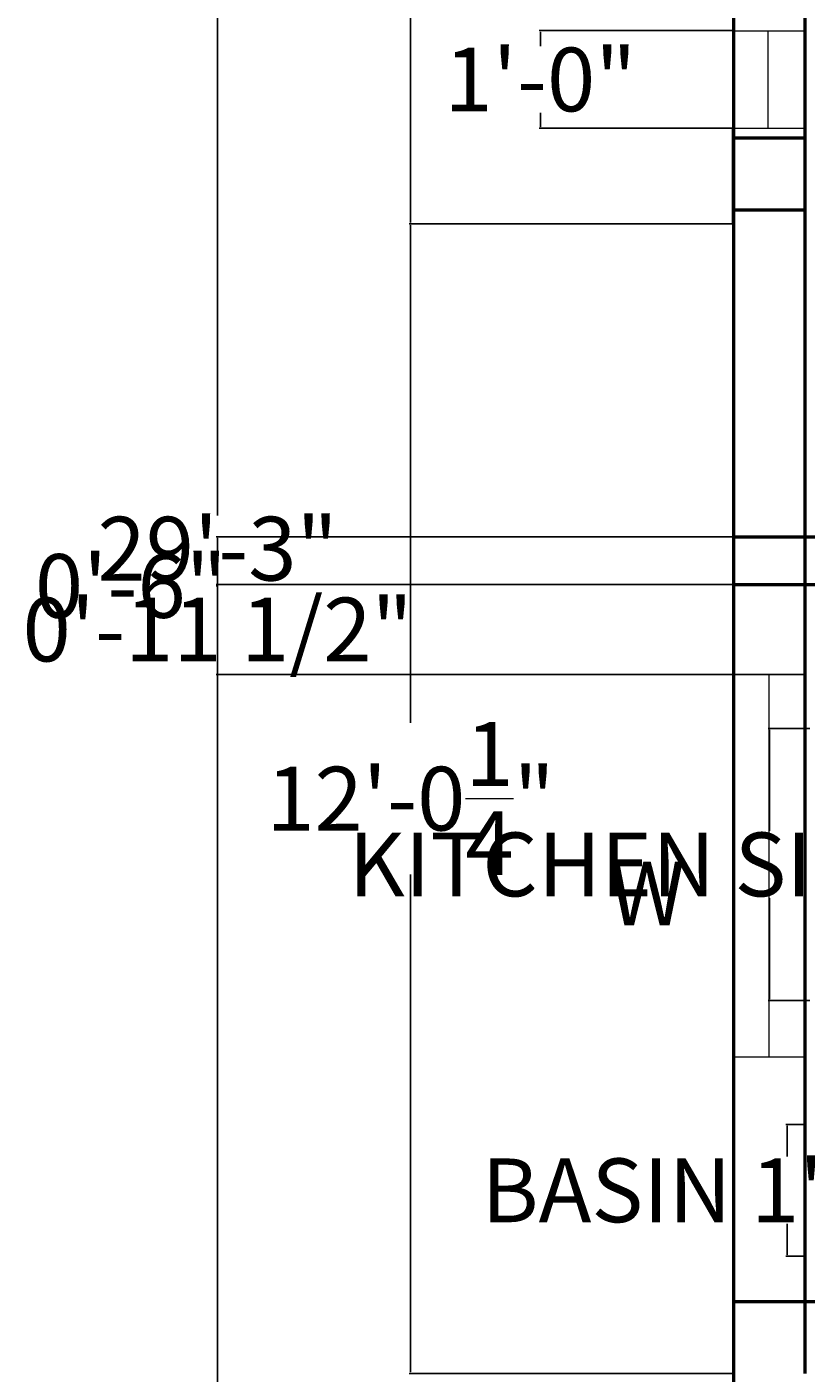
# Model space of a CAD drawing. Units: inches. Extents: x 1305 to 1889, y -508 to -5.
# Tile 2 of 8: x 1305 to 1403, y -389 to -220. Entities that reach past the tile are written whole.
import ezdxf

# ---------------------------------------------------------------- set-up
doc = ezdxf.new("R2010")
doc.units = ezdxf.units.IN
doc.header["$MEASUREMENT"] = 0
for name, color, linetype, lineweight in [('A-ANNO-DIMS', 2, 'Continuous', 18), ('A-ANNO-TEXT', 7, 'Continuous', 18), ('A-COLS', 7, 'Continuous', 50), ('A-GLAZ', 4, 'Continuous', 18), ('A-WALL', 7, 'Continuous', 50)]:
    doc.layers.add(name, color=color, linetype=linetype, lineweight=lineweight)
doc.styles.get("Standard").update_dxf_attribs({"font": 'arial.ttf', "height": 8})
doc.dimstyles.get("Standard").update_dxf_attribs({"dimtxt": 0.18, "dimasz": 0.18, "dimexe": 0.18, "dimexo": 0.0625, "dimgap": 0.09, "dimtad": 0, "dimtih": 1, "dimtoh": 1, "dimzin": 0, "dimdsep": 46, "dimlunit": 4, "dimtxsty": 'Standard', "dimcen": 0.09, "dimadec": 0, "dimazin": 0, "dimtfac": 1, "dimtofl": 0, "dimtmove": 0, "dimatfit": 3, "dimfxl": 1, "dimtolj": 1, "dimtzin": 0, "dimarcsym": 0})

# ---------------------------------------------------------------- blocks, each defined once
blk = doc.blocks.new('*D20')
at = {"layer": 'A-ANNO-DIMS', "color": 0, "lineweight": -2, "transparency": 16777216}
for p, q in [((1394.01, -110.24), (1353.36, -110.24)), ((1353.54, -110.42), (1353.54, -168.1)), ((1353.54, -244.8), (1353.54, -187.12)), ((1394.01, -244.98), (1353.36, -244.98))]:
    blk.add_line(p, q, dxfattribs=at)
at = {"layer": 'A-ANNO-DIMS', "color": 0, "transparency": 16777216}
for points in [[(1353.51, -110.42), (1353.57, -110.42), (1353.54, -110.24)], [(1353.51, -244.8), (1353.57, -244.8), (1353.54, -244.98)]]:
    blk.add_solid(points, dxfattribs=at)
at = {"layer": 'Defpoints', "color": 0, "transparency": 16777216}
for p in [(1394.07, -110.24), (1353.54, -244.98), (1394.07, -244.98)]:
    blk.add_point(p, dxfattribs=at)
at = {"layer": 'A-ANNO-DIMS', "color": 0, "transparency": 16777216, "insert": (1353.54, -177.61), "char_height": 8, "attachment_point": 5}
blk.add_mtext('\\A1;11\'-2{\\H1x;\\S3/4;}"', dxfattribs=at)
blk = doc.blocks.new('*D21')
at = {"layer": 'A-ANNO-DIMS', "color": 0, "lineweight": -2, "transparency": 16777216}
for p, q in [((1394.01, -244.98), (1353.36, -244.98)), ((1353.54, -245.16), (1353.54, -307.6)), ((1353.54, -389.06), (1353.54, -326.62)), ((1394.01, -389.24), (1353.36, -389.24))]:
    blk.add_line(p, q, dxfattribs=at)
at = {"layer": 'A-ANNO-DIMS', "color": 0, "transparency": 16777216}
for points in [[(1353.51, -245.16), (1353.57, -245.16), (1353.54, -244.98)], [(1353.51, -389.06), (1353.57, -389.06), (1353.54, -389.24)]]:
    blk.add_solid(points, dxfattribs=at)
at = {"layer": 'Defpoints', "color": 0, "transparency": 16777216}
for p in [(1394.07, -244.98), (1353.54, -389.24), (1394.07, -389.24)]:
    blk.add_point(p, dxfattribs=at)
at = {"layer": 'A-ANNO-DIMS', "color": 0, "transparency": 16777216, "insert": (1353.54, -317.11), "char_height": 8, "attachment_point": 5}
blk.add_mtext('\\A1;12\'-0{\\H1x;\\S1/4;}"', dxfattribs=at)
blk = doc.blocks.new('WIN-48IN')
for p, q in [((0, 9), (0, 0)), ((48, 9), (48, 0)), ((48, 4.5), (0, 4.5))]:
    blk.add_line(p, q)
blk = doc.blocks.new('COL-9X9')
blk.add_lwpolyline([(0, 0), (9, 0), (9, 9), (0, 9)], close=True)
blk = doc.blocks.new('*D34')
at = {"layer": 'A-ANNO-DIMS', "color": 0, "lineweight": -2, "transparency": 16777216}
for p, q in [((1403.25, -358), (1400.66, -358)), ((1400.84, -358.18), (1400.84, -362.04)), ((1400.84, -374.35), (1400.84, -370.49)), ((1403.25, -374.53), (1400.66, -374.53))]:
    blk.add_line(p, q, dxfattribs=at)
at = {"layer": 'A-ANNO-DIMS', "color": 0, "transparency": 16777216}
for points in [[(1400.81, -358.18), (1400.87, -358.18), (1400.84, -358)], [(1400.81, -374.35), (1400.87, -374.35), (1400.84, -374.53)]]:
    blk.add_solid(points, dxfattribs=at)
at = {"layer": 'Defpoints', "color": 0, "transparency": 16777216}
for p in [(1403.32, -358), (1400.84, -374.53), (1403.32, -374.53)]:
    blk.add_point(p, dxfattribs=at)
at = {"layer": 'A-ANNO-DIMS', "color": 0, "transparency": 16777216, "insert": (1400.84, -366.27), "char_height": 8, "attachment_point": 5}
blk.add_mtext('\\A1;BASIN 1\'-4 1/2"', dxfattribs=at)
blk = doc.blocks.new('*D44')
at = {"layer": 'A-ANNO-DIMS', "color": 0, "lineweight": -2, "transparency": 16777216}
for p, q in [((1403.68, -308.29), (1398.44, -308.29)), ((1398.62, -308.47), (1398.62, -321.14)), ((1398.62, -342.27), (1398.62, -329.59)), ((1403.68, -342.45), (1398.44, -342.45))]:
    blk.add_line(p, q, dxfattribs=at)
at = {"layer": 'A-ANNO-DIMS', "color": 0, "transparency": 16777216}
for points in [[(1398.59, -308.47), (1398.65, -308.47), (1398.62, -308.29)], [(1398.59, -342.27), (1398.65, -342.27), (1398.62, -342.45)]]:
    blk.add_solid(points, dxfattribs=at)
at = {"layer": 'Defpoints', "color": 0, "transparency": 16777216}
for p in [(1403.74, -308.29), (1398.62, -342.45), (1403.74, -342.45)]:
    blk.add_point(p, dxfattribs=at)
at = {"layer": 'A-ANNO-DIMS', "color": 0, "transparency": 16777216, "insert": (1398.62, -325.37), "char_height": 8, "attachment_point": 5}
blk.add_mtext('\\A1;KITCHEN SINK 2\'-10"', dxfattribs=at)
blk = doc.blocks.new('*D51')
at = {"layer": 'A-ANNO-DIMS', "color": 0, "lineweight": -2, "transparency": 16777216}
for p, q in [((1394.01, -110.24), (1329.13, -110.24)), ((1329.31, -110.42), (1329.31, -281.56)), ((1329.31, -461.06), (1329.31, -289.92)), ((1394.01, -461.24), (1329.13, -461.24))]:
    blk.add_line(p, q, dxfattribs=at)
at = {"layer": 'A-ANNO-DIMS', "color": 0, "transparency": 16777216}
for points in [[(1329.28, -110.42), (1329.34, -110.42), (1329.31, -110.24)], [(1329.28, -461.06), (1329.34, -461.06), (1329.31, -461.24)]]:
    blk.add_solid(points, dxfattribs=at)
at = {"layer": 'Defpoints', "color": 0, "transparency": 16777216}
for p in [(1394.07, -110.24), (1329.31, -461.24), (1394.07, -461.24)]:
    blk.add_point(p, dxfattribs=at)
at = {"layer": 'A-ANNO-DIMS', "color": 0, "transparency": 16777216, "insert": (1329.31, -285.74), "char_height": 8, "attachment_point": 5}
blk.add_mtext('\\A1;29\'-3"', dxfattribs=at)
blk = doc.blocks.new('*D62')
at = {"layer": 'A-ANNO-DIMS', "color": 0, "lineweight": -2, "transparency": 16777216}
for p, q in [((1505.01, -284.24), (1329.13, -284.24)), ((1329.31, -284.42), (1329.31, -290.06)), ((1505.01, -290.24), (1329.13, -290.24)), ((1329.31, -290.42), (1329.13, -290.42)), ((1329.31, -290.24), (1329.31, -290.42))]:
    blk.add_line(p, q, dxfattribs=at)
at = {"layer": 'A-ANNO-DIMS', "color": 0, "transparency": 16777216}
for points in [[(1329.28, -284.42), (1329.34, -284.42), (1329.31, -284.24)], [(1329.28, -290.06), (1329.34, -290.06), (1329.31, -290.24)]]:
    blk.add_solid(points, dxfattribs=at)
at = {"layer": 'Defpoints', "color": 0, "transparency": 16777216}
for p in [(1505.07, -284.24), (1329.31, -290.24), (1505.07, -290.24)]:
    blk.add_point(p, dxfattribs=at)
at = {"layer": 'A-ANNO-DIMS', "color": 0, "transparency": 16777216, "insert": (1318.41, -290.42), "char_height": 8, "attachment_point": 5}
blk.add_mtext('\\A1;0\'-6"', dxfattribs=at)
blk = doc.blocks.new('*D66')
at = {"layer": 'A-ANNO-DIMS', "color": 0, "lineweight": -2, "transparency": 16777216}
for p, q in [((1394.01, -290.24), (1329.13, -290.24)), ((1329.31, -290.42), (1329.31, -291.67)), ((1329.31, -301.37), (1329.31, -300.12)), ((1403.01, -301.55), (1329.13, -301.55))]:
    blk.add_line(p, q, dxfattribs=at)
at = {"layer": 'A-ANNO-DIMS', "color": 0, "transparency": 16777216}
for points in [[(1329.28, -290.42), (1329.34, -290.42), (1329.31, -290.24)], [(1329.28, -301.37), (1329.34, -301.37), (1329.31, -301.55)]]:
    blk.add_solid(points, dxfattribs=at)
at = {"layer": 'Defpoints', "color": 0, "transparency": 16777216}
for p in [(1394.07, -290.24), (1329.31, -301.55), (1403.07, -301.55)]:
    blk.add_point(p, dxfattribs=at)
at = {"layer": 'A-ANNO-DIMS', "color": 0, "transparency": 16777216, "insert": (1329.31, -295.89), "char_height": 8, "attachment_point": 5}
blk.add_mtext('\\A1;0\'-11 1/2"', dxfattribs=at)
blk = doc.blocks.new('*D73')
at = {"layer": 'A-ANNO-DIMS', "color": 0, "lineweight": -2, "transparency": 16777216}
for p, q in [((1394.01, -220.73), (1369.67, -220.73)), ((1369.85, -220.91), (1369.85, -222.68)), ((1369.85, -232.8), (1369.85, -231.03)), ((1394.01, -232.98), (1369.67, -232.98))]:
    blk.add_line(p, q, dxfattribs=at)
at = {"layer": 'A-ANNO-DIMS', "color": 0, "transparency": 16777216}
for points in [[(1369.82, -220.91), (1369.88, -220.91), (1369.85, -220.73)], [(1369.82, -232.8), (1369.88, -232.8), (1369.85, -232.98)]]:
    blk.add_solid(points, dxfattribs=at)
at = {"layer": 'Defpoints', "color": 0, "transparency": 16777216}
for p in [(1369.85, -220.73), (1394.07, -220.73), (1394.07, -232.98)]:
    blk.add_point(p, dxfattribs=at)
at = {"layer": 'A-ANNO-DIMS', "color": 0, "transparency": 16777216, "insert": (1369.85, -226.86), "char_height": 8, "attachment_point": 5}
blk.add_mtext('\\A1;1\'-0"', dxfattribs=at)

msp = doc.modelspace()

# ---------------------------------------------------------------- linework, layer by layer
at = {"layer": 'A-GLAZ'}
for p, q in [((1394.074, -220.734), (1403.074, -220.734)), ((1398.425, -220.734), (1398.425, -232.978)), ((1394.074, -232.978), (1403.074, -232.978))]:
    msp.add_line(p, q, dxfattribs=at)
at = {"layer": 'A-WALL'}
for p, q in [((1394.074, -110.239), (1394.074, -461.239)), ((1403.074, -110.239), (1403.074, -389.239)), ((1394.074, -244.978), (1394.074, -232.978)), ((1403.074, -232.978), (1403.074, -244.978)), ((1394.074, -284.239), (1505.074, -284.239)), ((1394.074, -290.239), (1505.074, -290.239)), ((1394.074, -380.239), (1547.074, -380.239))]:
    msp.add_line(p, q, dxfattribs=at)

# ---------------------------------------------------------------- block references
at = {"layer": 'A-COLS'}
msp.add_blockref('COL-9X9', (1394.108, -243.228), dxfattribs=at)
at = {"layer": 'A-GLAZ', "rotation": 269.9999999999999}
msp.add_blockref('WIN-48IN', (1394.074, -301.548), dxfattribs=at)

# ---------------------------------------------------------------- texts
at = {"layer": 'A-ANNO-TEXT', "insert": (1378.42, -325.014), "char_height": 8, "attachment_point": 1}
msp.add_mtext_dynamic_manual_height_columns('W', width=13.3749, gutter_width=40, heights=[0], dxfattribs=at)

# ---------------------------------------------------------------- dimensions: what is measured, and where the dimension line sits
at = {"layer": 'A-ANNO-DIMS'}
for base, p1, p2, override, picture, middle in [((1329.31, -461.239), (1394.074, -110.239), (1394.074, -461.239), {"dimdec": 1, "dimlfac": 1, "dimrnd": 0, "dimzin": 1, "dimdsep": 46, "dimlunit": 4, "dimfrac": 2}, '*D51', (1329.31, -285.739)), ((1353.535, -244.978), (1394.074, -110.239), (1394.074, -244.978), {"dimclrd": 0, "dimclre": 0, "dimclrt": 0}, '*D20', (1353.535, -177.608)), ((1369.849, -220.734), (1394.074, -232.978), (1394.074, -220.734), {"dimdec": 1, "dimlfac": 1, "dimrnd": 0, "dimzin": 1, "dimdsep": 46, "dimlunit": 4, "dimfrac": 2}, '*D73', (1369.849, -226.856)), ((1353.535, -389.239), (1394.074, -244.978), (1394.074, -389.239), {"dimclrd": 0, "dimclre": 0, "dimclrt": 0}, '*D21', (1353.535, -317.108)), ((1329.31, -301.547), (1394.074, -290.239), (1403.074, -301.547), {"dimdec": 1, "dimlfac": 1, "dimrnd": 0, "dimzin": 1, "dimdsep": 46, "dimlunit": 4, "dimfrac": 2}, '*D66', (1329.31, -295.893)), ((1329.31, -290.239), (1505.074, -284.239), (1505.074, -290.239), {"dimdec": 1, "dimlfac": 1, "dimrnd": 0, "dimzin": 1, "dimdsep": 46, "dimlunit": 4, "dimfrac": 2}, '*D62', (1318.407, -290.419))]:
    dim = msp.add_linear_dim(base=base, p1=p1, p2=p2, angle=90, dimstyle='Standard', override=override, dxfattribs=at)
    dim.commit()
    dim.dimension.update_dxf_attribs({"geometry": picture, "text_midpoint": middle})
for base, p1, p2, text, picture, middle in [((1398.618, -342.445), (1403.742, -308.29), (1403.742, -342.445), 'KITCHEN SINK <>', '*D44', (1398.618, -325.368)), ((1400.836, -374.535), (1403.316, -357.999), (1403.316, -374.535), 'BASIN <>', '*D34', (1400.836, -366.267))]:
    dim = msp.add_linear_dim(base=base, p1=p1, p2=p2, angle=270, text=text, dimstyle='Standard', override={"dimdec": 1, "dimlfac": 1, "dimrnd": 0, "dimzin": 1, "dimdsep": 46, "dimlunit": 4, "dimfrac": 2}, dxfattribs=at)
    dim.commit()
    dim.dimension.update_dxf_attribs({"geometry": picture, "text_midpoint": middle})

doc.saveas('drawing.dxf')
